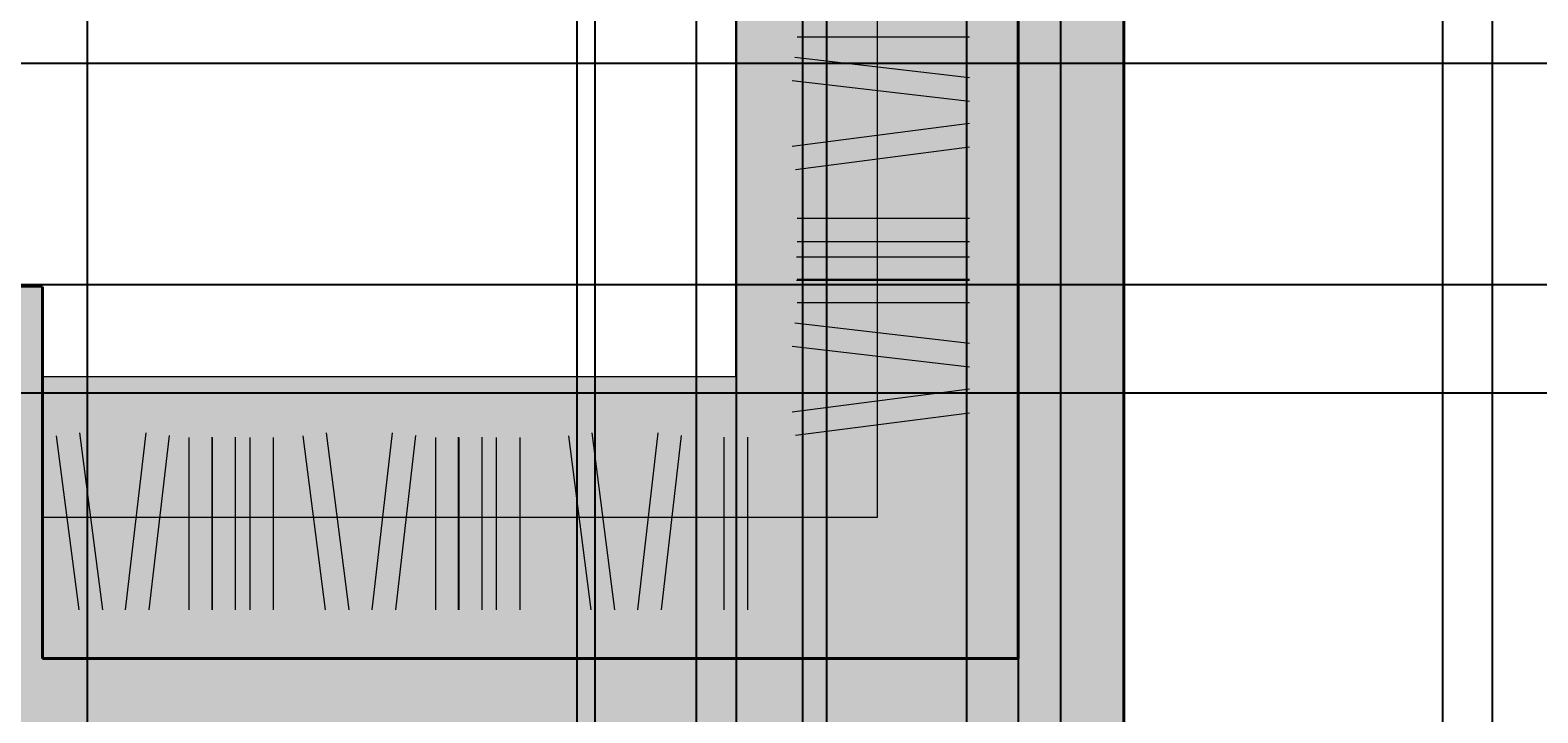
# Model space of a CAD drawing. Units: inches. Extents: x 818 to 1898, y 976 to 2364.
# Tile 42 of 96: x 1622 to 1750, y 1350 to 1409. Entities that reach past the tile are written whole.
import ezdxf

# ---------------------------------------------------------------- set-up
doc = ezdxf.new("R2010")
doc.units = ezdxf.units.IN
doc.header["$LTSCALE"] = 5
doc.header["$MEASUREMENT"] = 0
for name, color, linetype, lineweight in [('A-ANNO-DIMS', 2, 'Continuous', 18), ('A-DOOR', 3, 'Continuous', 25), ('A-FLOR-CASE', 8, 'Continuous', 18), ('A-FLOR-CASE-PATT', 33, 'Continuous', 9), ('A-WALL', 7, 'Continuous', 40)]:
    doc.layers.add(name, color=color, linetype=linetype, lineweight=lineweight)
doc.layers.add('A-WALL-PATT', color=251, linetype='Continuous', lineweight=13, true_color=0x636466)
doc.styles.get("Standard").update_dxf_attribs({"font": 'arial.ttf'})
doc.dimstyles.get("Standard").update_dxf_attribs({"dimtxt": 0.18, "dimasz": 0.18, "dimexe": 0.18, "dimexo": 0.0625, "dimgap": 0.09, "dimtad": 0, "dimtih": 1, "dimtoh": 1, "dimdec": 4, "dimzin": 0, "dimdsep": 46, "dimtxsty": 'Standard', "dimcen": 0.09, "dimadec": 0, "dimazin": 0, "dimtfac": 1, "dimtdec": 4, "dimtofl": 0, "dimtmove": 0, "dimatfit": 3, "dimfxl": 1, "dimtolj": 1, "dimtzin": 0, "dimarcsym": 0})

# ---------------------------------------------------------------- blocks, each defined once
blk = doc.blocks.new('*D71')
at = {"layer": 'A-ANNO-DIMS', "color": 0, "lineweight": -2, "ltscale": 5, "transparency": 16777216}
for p, q in [((1714.79, 2053.08), (1897.92, 2053.08)), ((1897.74, 2052.9), (1897.74, 1699.76)), ((1897.74, 1346.26), (1897.74, 1699.4)), ((1714.79, 1346.08), (1897.92, 1346.08))]:
    blk.add_line(p, q, dxfattribs=at)
at = {"layer": 'A-ANNO-DIMS', "color": 0, "ltscale": 5, "transparency": 16777216}
for points in [[(1897.71, 2052.9), (1897.77, 2052.9), (1897.74, 2053.08)], [(1897.71, 1346.26), (1897.77, 1346.26), (1897.74, 1346.08)]]:
    blk.add_solid(points, dxfattribs=at)
at = {"layer": 'Defpoints', "color": 0, "ltscale": 5, "transparency": 16777216}
for p in [(1714.73, 2053.08), (1897.74, 2053.08), (1714.73, 1346.08)]:
    blk.add_point(p, dxfattribs=at)
at = {"layer": 'A-ANNO-DIMS', "color": 0, "ltscale": 5, "transparency": 16777216, "insert": (1897.74, 1699.58), "char_height": 0.18, "attachment_point": 5}
blk.add_mtext('\\A1;707', dxfattribs=at)
blk = doc.blocks.new('*D102')
at = {"layer": 'A-ANNO-DIMS', "color": 0, "lineweight": -2, "ltscale": 5, "transparency": 16777216}
for p, q in [((1565.48, 1071.12), (1565.48, 2363.87)), ((1565.66, 2363.69), (1595.63, 2363.69)), ((1626.39, 2363.69), (1596.42, 2363.69)), ((1626.57, 1071.12), (1626.57, 2363.87))]:
    blk.add_line(p, q, dxfattribs=at)
at = {"layer": 'A-ANNO-DIMS', "color": 0, "ltscale": 5, "transparency": 16777216}
for points in [[(1565.66, 2363.72), (1565.66, 2363.66), (1565.48, 2363.69)], [(1626.39, 2363.72), (1626.39, 2363.66), (1626.57, 2363.69)]]:
    blk.add_solid(points, dxfattribs=at)
at = {"layer": 'Defpoints', "color": 0, "ltscale": 5, "transparency": 16777216}
for p in [(1626.57, 2363.69), (1565.48, 1071.06), (1626.57, 1071.06)]:
    blk.add_point(p, dxfattribs=at)
at = {"layer": 'A-ANNO-DIMS', "color": 0, "ltscale": 5, "transparency": 16777216, "insert": (1596.03, 2363.69), "char_height": 0.18, "attachment_point": 5}
blk.add_mtext('\\A1;61.09', dxfattribs=at)
blk = doc.blocks.new('*D103')
at = {"layer": 'A-ANNO-DIMS', "color": 0, "lineweight": -2, "ltscale": 5, "transparency": 16777216}
for p, q in [((1626.57, 1071.12), (1626.57, 2363.87)), ((1626.75, 2363.69), (1657.7, 2363.69)), ((1689.29, 2363.69), (1658.35, 2363.69)), ((1689.47, 1071.12), (1689.47, 2363.87))]:
    blk.add_line(p, q, dxfattribs=at)
at = {"layer": 'A-ANNO-DIMS', "color": 0, "ltscale": 5, "transparency": 16777216}
for points in [[(1626.75, 2363.72), (1626.75, 2363.66), (1626.57, 2363.69)], [(1689.29, 2363.72), (1689.29, 2363.66), (1689.47, 2363.69)]]:
    blk.add_solid(points, dxfattribs=at)
at = {"layer": 'Defpoints', "color": 0, "ltscale": 5, "transparency": 16777216}
for p in [(1689.47, 2363.69), (1626.57, 1071.06), (1689.47, 1071.06)]:
    blk.add_point(p, dxfattribs=at)
at = {"layer": 'A-ANNO-DIMS', "color": 0, "ltscale": 5, "transparency": 16777216, "insert": (1658.02, 2363.69), "char_height": 0.18, "attachment_point": 5}
blk.add_mtext('\\A1;62.9', dxfattribs=at)
blk = doc.blocks.new('*D104')
at = {"layer": 'A-ANNO-DIMS', "color": 0, "lineweight": -2, "ltscale": 5, "transparency": 16777216}
for p, q in [((1689.47, 1071.12), (1689.47, 2363.87)), ((1689.65, 2363.69), (1717.4, 2363.69)), ((1745.9, 2363.69), (1718.15, 2363.69)), ((1746.08, 1071.12), (1746.08, 2363.87))]:
    blk.add_line(p, q, dxfattribs=at)
at = {"layer": 'A-ANNO-DIMS', "color": 0, "ltscale": 5, "transparency": 16777216}
for points in [[(1689.65, 2363.72), (1689.65, 2363.66), (1689.47, 2363.69)], [(1745.9, 2363.72), (1745.9, 2363.66), (1746.08, 2363.69)]]:
    blk.add_solid(points, dxfattribs=at)
at = {"layer": 'Defpoints', "color": 0, "ltscale": 5, "transparency": 16777216}
for p in [(1746.08, 2363.69), (1689.47, 1071.06), (1746.08, 1071.06)]:
    blk.add_point(p, dxfattribs=at)
at = {"layer": 'A-ANNO-DIMS', "color": 0, "ltscale": 5, "transparency": 16777216, "insert": (1717.78, 2363.69), "char_height": 0.18, "attachment_point": 5}
blk.add_mtext('\\A1;56.61', dxfattribs=at)
blk = doc.blocks.new('*D112')
at = {"layer": 'A-ANNO-DIMS', "color": 0, "lineweight": -2, "ltscale": 5, "transparency": 16777216}
for p, q in [((1135.27, 1405.71), (1897.92, 1405.71)), ((1897.74, 1405.53), (1897.74, 1396.48)), ((1897.74, 1387.07), (1897.74, 1396.12)), ((1135.27, 1386.89), (1897.92, 1386.89))]:
    blk.add_line(p, q, dxfattribs=at)
at = {"layer": 'A-ANNO-DIMS', "color": 0, "ltscale": 5, "transparency": 16777216}
for points in [[(1897.71, 1405.53), (1897.77, 1405.53), (1897.74, 1405.71)], [(1897.71, 1387.07), (1897.77, 1387.07), (1897.74, 1386.89)]]:
    blk.add_solid(points, dxfattribs=at)
at = {"layer": 'Defpoints', "color": 0, "ltscale": 5, "transparency": 16777216}
for p in [(1135.21, 1405.71), (1135.21, 1386.89), (1897.74, 1386.89)]:
    blk.add_point(p, dxfattribs=at)
at = {"layer": 'A-ANNO-DIMS', "color": 0, "ltscale": 5, "transparency": 16777216, "insert": (1897.74, 1396.3), "char_height": 0.18, "attachment_point": 5}
blk.add_mtext('\\A1;18.824', dxfattribs=at)
blk = doc.blocks.new('*D115')
at = {"layer": 'A-ANNO-DIMS', "color": 0, "lineweight": -2, "ltscale": 5, "transparency": 16777216}
for p, q in [((1766.29, 1377.66), (818.03, 1377.66)), ((818.21, 1377.48), (818.21, 1338.26)), ((818.21, 1298.68), (818.21, 1337.9)), ((1766.29, 1298.5), (818.03, 1298.5))]:
    blk.add_line(p, q, dxfattribs=at)
at = {"layer": 'A-ANNO-DIMS', "color": 0, "ltscale": 5, "transparency": 16777216}
for points in [[(818.18, 1377.48), (818.24, 1377.48), (818.21, 1377.66)], [(818.18, 1298.68), (818.24, 1298.68), (818.21, 1298.5)]]:
    blk.add_solid(points, dxfattribs=at)
at = {"layer": 'Defpoints', "color": 0, "ltscale": 5, "transparency": 16777216}
for p in [(818.21, 1377.66), (1766.35, 1377.66), (1766.35, 1298.5)]:
    blk.add_point(p, dxfattribs=at)
at = {"layer": 'A-ANNO-DIMS', "color": 0, "ltscale": 5, "transparency": 16777216, "insert": (818.21, 1338.08), "char_height": 0.18, "attachment_point": 5}
blk.add_mtext('\\A1;79.15', dxfattribs=at)
blk = doc.blocks.new('*D116')
at = {"layer": 'A-ANNO-DIMS', "color": 0, "lineweight": -2, "ltscale": 5, "transparency": 16777216}
for p, q in [((1766.29, 1456.81), (818.03, 1456.81)), ((818.21, 1456.63), (818.21, 1417.41)), ((818.21, 1377.84), (818.21, 1417.05)), ((1766.29, 1377.66), (818.03, 1377.66))]:
    blk.add_line(p, q, dxfattribs=at)
at = {"layer": 'A-ANNO-DIMS', "color": 0, "ltscale": 5, "transparency": 16777216}
for points in [[(818.18, 1456.63), (818.24, 1456.63), (818.21, 1456.81)], [(818.18, 1377.84), (818.24, 1377.84), (818.21, 1377.66)]]:
    blk.add_solid(points, dxfattribs=at)
at = {"layer": 'Defpoints', "color": 0, "ltscale": 5, "transparency": 16777216}
for p in [(818.21, 1456.81), (1766.35, 1456.81), (1766.35, 1377.66)]:
    blk.add_point(p, dxfattribs=at)
at = {"layer": 'A-ANNO-DIMS', "color": 0, "ltscale": 5, "transparency": 16777216, "insert": (818.21, 1417.23), "char_height": 0.18, "attachment_point": 5}
blk.add_mtext('\\A1;79.15', dxfattribs=at)
blk = doc.blocks.new('*D154')
at = {"layer": 'A-ANNO-DIMS', "color": 0, "lineweight": -2, "ltscale": 5, "transparency": 16777216}
for p, q in [((1701.37, 1290.14), (1701.37, 2363.87)), ((1701.55, 2363.69), (1705.22, 2363.69)), ((1709.19, 2363.69), (1705.52, 2363.69)), ((1709.37, 1298.14), (1709.37, 2363.87))]:
    blk.add_line(p, q, dxfattribs=at)
at = {"layer": 'A-ANNO-DIMS', "color": 0, "ltscale": 5, "transparency": 16777216}
for points in [[(1701.55, 2363.72), (1701.55, 2363.66), (1701.37, 2363.69)], [(1709.19, 2363.72), (1709.19, 2363.66), (1709.37, 2363.69)]]:
    blk.add_solid(points, dxfattribs=at)
at = {"layer": 'Defpoints', "color": 0, "ltscale": 5, "transparency": 16777216}
for p in [(1709.37, 2363.69), (1709.37, 1298.08), (1701.37, 1290.08)]:
    blk.add_point(p, dxfattribs=at)
at = {"layer": 'A-ANNO-DIMS', "color": 0, "ltscale": 5, "transparency": 16777216, "insert": (1705.37, 2363.69), "char_height": 0.18, "attachment_point": 5}
blk.add_mtext('\\A1;8', dxfattribs=at)
blk = doc.blocks.new('*D178')
at = {"layer": 'A-ANNO-DIMS', "color": 0, "lineweight": -2, "ltscale": 5, "transparency": 16777216}
for p, q in [((1669.73, 1600.02), (1669.73, 975.66)), ((1705.73, 1600.02), (1705.73, 975.66)), ((1669.91, 975.84), (1687.51, 975.84)), ((1705.55, 975.84), (1687.94, 975.84))]:
    blk.add_line(p, q, dxfattribs=at)
at = {"layer": 'A-ANNO-DIMS', "color": 0, "ltscale": 5, "transparency": 16777216}
for points in [[(1669.91, 975.87), (1669.91, 975.81), (1669.73, 975.84)], [(1705.55, 975.87), (1705.55, 975.81), (1705.73, 975.84)]]:
    blk.add_solid(points, dxfattribs=at)
at = {"layer": 'Defpoints', "color": 0, "ltscale": 5, "transparency": 16777216}
for p in [(1669.73, 1600.08), (1705.73, 1600.08), (1705.73, 975.84)]:
    blk.add_point(p, dxfattribs=at)
at = {"layer": 'A-ANNO-DIMS', "color": 0, "ltscale": 5, "transparency": 16777216, "insert": (1687.73, 975.84), "char_height": 0.18, "attachment_point": 5}
blk.add_mtext('\\A1;36', dxfattribs=at)
blk = doc.blocks.new('*D180')
at = {"layer": 'A-ANNO-DIMS', "color": 0, "lineweight": -2, "ltscale": 5, "transparency": 16777216}
for p, q in [((1599.73, 1639.52), (1599.73, 975.66)), ((1669.73, 1639.52), (1669.73, 975.66)), ((1599.91, 975.84), (1634.51, 975.84)), ((1669.55, 975.84), (1634.94, 975.84))]:
    blk.add_line(p, q, dxfattribs=at)
at = {"layer": 'A-ANNO-DIMS', "color": 0, "ltscale": 5, "transparency": 16777216}
for points in [[(1599.91, 975.87), (1599.91, 975.81), (1599.73, 975.84)], [(1669.55, 975.87), (1669.55, 975.81), (1669.73, 975.84)]]:
    blk.add_solid(points, dxfattribs=at)
at = {"layer": 'Defpoints', "color": 0, "ltscale": 5, "transparency": 16777216}
for p in [(1599.73, 1639.58), (1669.73, 1639.58), (1669.73, 975.84)]:
    blk.add_point(p, dxfattribs=at)
at = {"layer": 'A-ANNO-DIMS', "color": 0, "ltscale": 5, "transparency": 16777216, "insert": (1634.73, 975.84), "char_height": 0.18, "attachment_point": 5}
blk.add_mtext('\\A1;70', dxfattribs=at)
blk = doc.blocks.new('*D183')
at = {"layer": 'A-ANNO-DIMS', "color": 0, "lineweight": -2, "ltscale": 5, "transparency": 16777216}
for p, q in [((1714.73, 1545.02), (1714.73, 975.66)), ((1741.84, 1545.02), (1741.84, 975.66)), ((1714.91, 975.84), (1727.82, 975.84)), ((1741.66, 975.84), (1728.75, 975.84))]:
    blk.add_line(p, q, dxfattribs=at)
at = {"layer": 'A-ANNO-DIMS', "color": 0, "ltscale": 5, "transparency": 16777216}
for points in [[(1714.91, 975.87), (1714.91, 975.81), (1714.73, 975.84)], [(1741.66, 975.87), (1741.66, 975.81), (1741.84, 975.84)]]:
    blk.add_solid(points, dxfattribs=at)
at = {"layer": 'Defpoints', "color": 0, "ltscale": 5, "transparency": 16777216}
for p in [(1714.73, 1545.08), (1741.84, 1545.08), (1741.84, 975.84)]:
    blk.add_point(p, dxfattribs=at)
at = {"layer": 'A-ANNO-DIMS', "color": 0, "ltscale": 5, "transparency": 16777216, "insert": (1728.28, 975.84), "char_height": 0.18, "attachment_point": 5}
blk.add_mtext('\\A1;27.116', dxfattribs=at)
blk = doc.blocks.new('*D188')
at = {"layer": 'A-ANNO-DIMS', "color": 0, "lineweight": -2, "ltscale": 5, "transparency": 16777216}
for p, q in [((1714.79, 1545.08), (1897.92, 1545.08)), ((1897.74, 1544.9), (1897.74, 1445.76)), ((1897.74, 1346.26), (1897.74, 1445.4)), ((1714.79, 1346.08), (1897.92, 1346.08))]:
    blk.add_line(p, q, dxfattribs=at)
at = {"layer": 'A-ANNO-DIMS', "color": 0, "ltscale": 5, "transparency": 16777216}
for points in [[(1897.71, 1544.9), (1897.77, 1544.9), (1897.74, 1545.08)], [(1897.71, 1346.26), (1897.77, 1346.26), (1897.74, 1346.08)]]:
    blk.add_solid(points, dxfattribs=at)
at = {"layer": 'Defpoints', "color": 0, "ltscale": 5, "transparency": 16777216}
for p in [(1714.73, 1545.08), (1897.74, 1545.08), (1714.73, 1346.08)]:
    blk.add_point(p, dxfattribs=at)
at = {"layer": 'A-ANNO-DIMS', "color": 0, "ltscale": 5, "transparency": 16777216, "insert": (1897.74, 1445.58), "char_height": 0.18, "attachment_point": 5}
blk.add_mtext('\\A1;199', dxfattribs=at)
blk = doc.blocks.new('*D195')
at = {"layer": 'A-ANNO-DIMS', "color": 0, "lineweight": -2, "ltscale": 5, "transparency": 16777216}
for p, q in [((1681.73, 1379.14), (1681.73, 2363.87)), ((1681.91, 2363.69), (1693.51, 2363.69)), ((1705.55, 2363.69), (1693.95, 2363.69)), ((1705.73, 1355.14), (1705.73, 2363.87))]:
    blk.add_line(p, q, dxfattribs=at)
at = {"layer": 'A-ANNO-DIMS', "color": 0, "ltscale": 5, "transparency": 16777216}
for points in [[(1681.91, 2363.72), (1681.91, 2363.66), (1681.73, 2363.69)], [(1705.55, 2363.72), (1705.55, 2363.66), (1705.73, 2363.69)]]:
    blk.add_solid(points, dxfattribs=at)
at = {"layer": 'Defpoints', "color": 0, "ltscale": 5, "transparency": 16777216}
for p in [(1705.73, 2363.69), (1681.73, 1379.08), (1705.73, 1355.08)]:
    blk.add_point(p, dxfattribs=at)
at = {"layer": 'A-ANNO-DIMS', "color": 0, "ltscale": 5, "transparency": 16777216, "insert": (1693.73, 2363.69), "char_height": 0.18, "attachment_point": 5}
blk.add_mtext('\\A1;24', dxfattribs=at)
blk = doc.blocks.new('*D198')
at = {"layer": 'A-ANNO-DIMS', "color": 0, "lineweight": -2, "ltscale": 5, "transparency": 16777216}
for p, q in [((1741.84, 1545.02), (1741.84, 975.66)), ((1430.73, 1346.02), (1430.73, 975.66)), ((1430.91, 975.84), (1585.91, 975.84)), ((1741.66, 975.84), (1586.66, 975.84))]:
    blk.add_line(p, q, dxfattribs=at)
at = {"layer": 'A-ANNO-DIMS', "color": 0, "ltscale": 5, "transparency": 16777216}
for points in [[(1430.91, 975.87), (1430.91, 975.81), (1430.73, 975.84)], [(1741.66, 975.87), (1741.66, 975.81), (1741.84, 975.84)]]:
    blk.add_solid(points, dxfattribs=at)
at = {"layer": 'Defpoints', "color": 0, "ltscale": 5, "transparency": 16777216}
for p in [(1741.84, 1545.08), (1430.73, 1346.08), (1741.84, 975.84)]:
    blk.add_point(p, dxfattribs=at)
at = {"layer": 'A-ANNO-DIMS', "color": 0, "ltscale": 5, "transparency": 16777216, "insert": (1586.28, 975.84), "char_height": 0.18, "attachment_point": 5}
blk.add_mtext('\\A1;311.1', dxfattribs=at)
blk = doc.blocks.new('*D199')
at = {"layer": 'A-ANNO-DIMS', "color": 0, "lineweight": -2, "ltscale": 5, "transparency": 16777216}
for p, q in [((1559.79, 1687.08), (1897.92, 1687.08)), ((1897.74, 1686.9), (1897.74, 1513.15)), ((1897.74, 1339.05), (1897.74, 1512.79)), ((1660.38, 1338.87), (1897.92, 1338.87))]:
    blk.add_line(p, q, dxfattribs=at)
at = {"layer": 'A-ANNO-DIMS', "color": 0, "ltscale": 5, "transparency": 16777216}
for points in [[(1897.71, 1686.9), (1897.77, 1686.9), (1897.74, 1687.08)], [(1897.71, 1339.05), (1897.77, 1339.05), (1897.74, 1338.87)]]:
    blk.add_solid(points, dxfattribs=at)
at = {"layer": 'Defpoints', "color": 0, "ltscale": 5, "transparency": 16777216}
for p in [(1559.73, 1687.08), (1897.74, 1687.08), (1660.31, 1338.87)]:
    blk.add_point(p, dxfattribs=at)
at = {"layer": 'A-ANNO-DIMS', "color": 0, "ltscale": 5, "transparency": 16777216, "insert": (1897.74, 1512.97), "char_height": 0.18, "attachment_point": 5}
blk.add_mtext('\\A1;348.2', dxfattribs=at)
blk = doc.blocks.new('*D200')
at = {"layer": 'A-ANNO-DIMS', "color": 0, "lineweight": -2, "ltscale": 5, "transparency": 16777216}
for p, q in [((1678.33, 1477.36), (1678.33, 975.66)), ((1705.73, 1477.36), (1705.73, 975.66)), ((1678.51, 975.84), (1691.56, 975.84)), ((1705.55, 975.84), (1692.49, 975.84))]:
    blk.add_line(p, q, dxfattribs=at)
at = {"layer": 'A-ANNO-DIMS', "color": 0, "ltscale": 5, "transparency": 16777216}
for points in [[(1678.51, 975.87), (1678.51, 975.81), (1678.33, 975.84)], [(1705.55, 975.87), (1705.55, 975.81), (1705.73, 975.84)]]:
    blk.add_solid(points, dxfattribs=at)
at = {"layer": 'Defpoints', "color": 0, "ltscale": 5, "transparency": 16777216}
for p in [(1678.33, 1477.43), (1705.73, 1477.43), (1705.73, 975.84)]:
    blk.add_point(p, dxfattribs=at)
at = {"layer": 'A-ANNO-DIMS', "color": 0, "ltscale": 5, "transparency": 16777216, "insert": (1692.03, 975.84), "char_height": 0.18, "attachment_point": 5}
blk.add_mtext('\\A1;27.395', dxfattribs=at)
blk = doc.blocks.new('*D212')
at = {"layer": 'A-ANNO-DIMS', "color": 0, "lineweight": -2, "ltscale": 5, "transparency": 16777216}
for p, q in [((1681.73, 1900.02), (1681.73, 975.66)), ((1705.73, 1876.02), (1705.73, 975.66)), ((1681.91, 975.84), (1693.51, 975.84)), ((1705.55, 975.84), (1693.95, 975.84))]:
    blk.add_line(p, q, dxfattribs=at)
at = {"layer": 'A-ANNO-DIMS', "color": 0, "ltscale": 5, "transparency": 16777216}
for points in [[(1681.91, 975.87), (1681.91, 975.81), (1681.73, 975.84)], [(1705.55, 975.87), (1705.55, 975.81), (1705.73, 975.84)]]:
    blk.add_solid(points, dxfattribs=at)
at = {"layer": 'Defpoints', "color": 0, "ltscale": 5, "transparency": 16777216}
for p in [(1681.73, 1900.08), (1705.73, 1876.08), (1705.73, 975.84)]:
    blk.add_point(p, dxfattribs=at)
at = {"layer": 'A-ANNO-DIMS', "color": 0, "ltscale": 5, "transparency": 16777216, "insert": (1693.73, 975.84), "char_height": 0.18, "attachment_point": 5}
blk.add_mtext('\\A1;24', dxfattribs=at)
blk = doc.blocks.new('*D214')
at = {"layer": 'A-ANNO-DIMS', "color": 0, "lineweight": -2, "ltscale": 5, "transparency": 16777216}
for p, q in [((1511.73, 1687.02), (1511.73, 975.66)), ((1714.73, 1687.02), (1714.73, 975.66)), ((1511.91, 975.84), (1612.93, 975.84)), ((1714.55, 975.84), (1613.52, 975.84))]:
    blk.add_line(p, q, dxfattribs=at)
at = {"layer": 'A-ANNO-DIMS', "color": 0, "ltscale": 5, "transparency": 16777216}
for points in [[(1511.91, 975.87), (1511.91, 975.81), (1511.73, 975.84)], [(1714.55, 975.87), (1714.55, 975.81), (1714.73, 975.84)]]:
    blk.add_solid(points, dxfattribs=at)
at = {"layer": 'Defpoints', "color": 0, "ltscale": 5, "transparency": 16777216}
for p in [(1511.73, 1687.08), (1714.73, 1687.08), (1714.73, 975.84)]:
    blk.add_point(p, dxfattribs=at)
at = {"layer": 'A-ANNO-DIMS', "color": 0, "ltscale": 5, "transparency": 16777216, "insert": (1613.23, 975.84), "char_height": 0.18, "attachment_point": 5}
blk.add_mtext('\\A1;203', dxfattribs=at)
blk = doc.blocks.new('*D221')
at = {"layer": 'A-ANNO-DIMS', "color": 0, "lineweight": -2, "ltscale": 5, "transparency": 16777216}
for p, q in [((1668.18, 1696.02), (1668.18, 975.66)), ((1705.73, 1696.02), (1705.73, 975.66)), ((1668.36, 975.84), (1686.56, 975.84)), ((1705.55, 975.84), (1687.35, 975.84))]:
    blk.add_line(p, q, dxfattribs=at)
at = {"layer": 'A-ANNO-DIMS', "color": 0, "ltscale": 5, "transparency": 16777216}
for points in [[(1668.36, 975.87), (1668.36, 975.81), (1668.18, 975.84)], [(1705.55, 975.87), (1705.55, 975.81), (1705.73, 975.84)]]:
    blk.add_solid(points, dxfattribs=at)
at = {"layer": 'Defpoints', "color": 0, "ltscale": 5, "transparency": 16777216}
for p in [(1668.18, 1696.08), (1705.73, 1696.08), (1705.73, 975.84)]:
    blk.add_point(p, dxfattribs=at)
at = {"layer": 'A-ANNO-DIMS', "color": 0, "ltscale": 5, "transparency": 16777216, "insert": (1686.95, 975.84), "char_height": 0.18, "attachment_point": 5}
blk.add_mtext('\\A1;37.54', dxfattribs=at)
blk = doc.blocks.new('*D228')
at = {"layer": 'A-ANNO-DIMS', "color": 0, "lineweight": -2, "ltscale": 5, "transparency": 16777216}
for p, q in [((1687.39, 1802.02), (1687.39, 975.66)), ((1705.73, 1802.02), (1705.73, 975.66)), ((1687.57, 975.84), (1696.17, 975.84)), ((1705.55, 975.84), (1696.94, 975.84))]:
    blk.add_line(p, q, dxfattribs=at)
at = {"layer": 'A-ANNO-DIMS', "color": 0, "ltscale": 5, "transparency": 16777216}
for points in [[(1687.57, 975.87), (1687.57, 975.81), (1687.39, 975.84)], [(1705.55, 975.87), (1705.55, 975.81), (1705.73, 975.84)]]:
    blk.add_solid(points, dxfattribs=at)
at = {"layer": 'Defpoints', "color": 0, "ltscale": 5, "transparency": 16777216}
for p in [(1687.39, 1802.08), (1705.73, 1802.08), (1705.73, 975.84)]:
    blk.add_point(p, dxfattribs=at)
at = {"layer": 'A-ANNO-DIMS', "color": 0, "ltscale": 5, "transparency": 16777216, "insert": (1696.56, 975.84), "char_height": 0.18, "attachment_point": 5}
blk.add_mtext('\\A1;18.33', dxfattribs=at)
blk = doc.blocks.new('*D267')
at = {"layer": 'A-ANNO-DIMS', "color": 0, "lineweight": -2, "ltscale": 5, "transparency": 16777216}
for p, q in [((1714.73, 1687.02), (1714.73, 975.66)), ((1741.84, 1687.02), (1741.84, 975.66)), ((1714.91, 975.84), (1727.82, 975.84)), ((1741.66, 975.84), (1728.75, 975.84))]:
    blk.add_line(p, q, dxfattribs=at)
at = {"layer": 'A-ANNO-DIMS', "color": 0, "ltscale": 5, "transparency": 16777216}
for points in [[(1714.91, 975.87), (1714.91, 975.81), (1714.73, 975.84)], [(1741.66, 975.87), (1741.66, 975.81), (1741.84, 975.84)]]:
    blk.add_solid(points, dxfattribs=at)
at = {"layer": 'Defpoints', "color": 0, "ltscale": 5, "transparency": 16777216}
for p in [(1714.73, 1687.08), (1741.84, 1687.08), (1741.84, 975.84)]:
    blk.add_point(p, dxfattribs=at)
at = {"layer": 'A-ANNO-DIMS', "color": 0, "ltscale": 5, "transparency": 16777216, "insert": (1728.28, 975.84), "char_height": 0.18, "attachment_point": 5}
blk.add_mtext('\\A1;27.116', dxfattribs=at)

msp = doc.modelspace()

# ---------------------------------------------------------------- hatches: boundary and pattern name
at = {"layer": 'A-FLOR-CASE-PATT', "ltscale": 5}
h = msp.add_hatch(color=256, dxfattribs=at)
h.dxf.hatch_style = 1
h.paths.add_polyline_path([(1705.7251, 1941.0782), (1681.7251, 1941.0782), (1681.7251, 1900.0782), (1599.7251, 1900.0782), (1599.7251, 1876.0782), (1705.7251, 1876.0782)])
h.paths.add_polyline_path([(1457.7252, 1409.1177), (1457.7252, 1526.6712), (1439.7252, 1526.6712), (1439.7252, 1457.5313), (1446.3307, 1457.5313), (1446.3307, 1468.9514), (1446.8307, 1470.665), (1446.8307, 1469.665), (1446.8307, 1468.9514), (1446.8307, 1456.8361), (1446.8307, 1444.7258), (1446.8307, 1443.3338), (1446.3307, 1444.7258), (1446.3307, 1456.8361), (1439.7252, 1456.8361), (1439.7252, 1355.0782), (1463.7252, 1355.0782), (1463.7252, 1367.3287), (1458.0475, 1367.3287, -0.23606798), (1457.0475, 1369.3287), (1456.0475, 1369.3287, -0.11764706), (1456.0475, 1386.3287), (1457.0475, 1386.3287, -0.23606798), (1458.0475, 1388.3287), (1463.7252, 1388.3287), (1463.7252, 1389.3211)])
h.paths.add_polyline_path([(1341.2593, 1534.0782), (1246.9377, 1534.0782), (1246.9377, 1510.0782), (1341.2593, 1510.0782)])
h.paths.add_polyline_path([(1288.8272, 1519.927), (1289.8272, 1519.927), (1290.5408, 1519.927), (1302.6561, 1519.927), (1314.7664, 1519.927), (1316.1584, 1519.927), (1314.7664, 1519.427), (1302.6561, 1519.427), (1302.6561, 1512.8214), (1301.9609, 1512.8214), (1301.9609, 1519.427), (1290.5408, 1519.427)], flags=16)
h.paths.add_polyline_path([(1377.7791, 1867.0782), (1344.5531, 1867.0782), (1344.5531, 1860.4726), (1355.9731, 1860.4726), (1357.6867, 1859.9726), (1356.6867, 1859.9726), (1355.9731, 1859.9726), (1343.8579, 1859.9726), (1331.7475, 1859.9726), (1330.3556, 1859.9726), (1331.7475, 1860.4726), (1343.8579, 1860.4726), (1343.8579, 1867.0782), (1311.3271, 1867.0782), (1311.3271, 1853.7496), (1377.7791, 1853.7496)])
h.paths.add_polyline_path([(1301.148, 1610.7299, -0.46196039), (1314.4882, 1599.3725, -0.19222541), (1311.3254, 1591.4497, 0.54791519), (1336.8832, 1607.7707, 0.92061359)])
h.paths.add_polyline_path([(1370.719, 1780.5695, 1), (1332.478, 1780.5695, 1)])
h.paths.add_polyline_path([(1705.7251, 1463.0782), (1681.7251, 1463.0782), (1681.7251, 1379.0782), (1622.7252, 1379.0782), (1622.7252, 1355.0782), (1705.7251, 1355.0782)])
h.paths.add_polyline_path([(1658.1052, 1359.2188), (1658.1786, 1359.2188), (1658.1786, 1373.8763), (1658.1052, 1373.9202)], flags=16)
h.paths.add_polyline_path([(1686.9271, 1409.9311), (1686.8832, 1409.8578), (1701.5845, 1409.8578), (1701.5845, 1409.9311)], flags=16)
h.paths.add_polyline_path([(1637.1266, 1359.2188), (1637.2, 1359.2188), (1637.2, 1373.8763), (1637.1266, 1373.9202)], flags=16)
at = {"layer": 'A-WALL-PATT', "ltscale": 5}
h = msp.add_hatch(color=256, dxfattribs=at)
h.dxf.hatch_style = 1
h.paths.add_polyline_path([(1714.7251, 1521.0782), (1705.7251, 1521.0782), (1705.7251, 1467.0782), (1654.7252, 1467.0782), (1654.7252, 1463.0782), (1705.7251, 1463.0782), (1705.7251, 1355.0782), (1622.7252, 1355.0782), (1622.7252, 1379.0782), (1622.7252, 1386.6857), (1616.7252, 1386.6857), (1616.7252, 1355.0782), (1490.9163, 1355.0782), (1490.9163, 1346.0782), (1544.7605, 1346.0782), (1544.6132, 1346.8783), (1544.6729, 1346.84), (1544.6299, 1346.7874), (1544.7605, 1346.0782), (1555.1299, 1346.0782), (1555.1299, 1341.5528), (1556.1599, 1340.8639), (1556.5281, 1338.8654), (1660.3141, 1338.8654), (1660.3141, 1346.0782), (1705.7251, 1346.0782), (1705.7251, 1345.0768), (1705.8704, 1344.58), (1705.7251, 1344.3933), (1705.7251, 1334.9904), (1705.8704, 1334.4936), (1705.7251, 1334.3068), (1705.7251, 1316.2253), (1707.3573, 1316.7694), (1707.3847, 1316.8046), (1707.3807, 1316.7771), (1705.7251, 1316.2253), (1705.7251, 1314.1392), (1705.7251, 1312.0957), (1705.8703, 1312.0739), (1705.7251, 1311.8873), (1705.7251, 1310.7121), (1706.5603, 1307.9282), (1707.8887, 1307.1831), (1714.7251, 1307.1831), (1714.7251, 1346.0782)])

# ---------------------------------------------------------------- linework, layer by layer
at = {"layer": 'A-DOOR'}
msp.add_line((1622.7252, 1386.6857), (1616.7252, 1386.6857), dxfattribs=at)
at = {"layer": 'A-FLOR-CASE'}
for p, q in [((1681.7251, 1463.0782), (1681.7251, 1379.0782)), ((1701.5845, 1407.9311), (1686.9271, 1407.9311)), ((1686.7478, 1406.2264), (1701.5845, 1404.5006)), ((1686.5168, 1404.2398), (1701.5845, 1402.4871)), ((1701.5845, 1400.5839), (1686.5199, 1398.6332)), ((1701.5845, 1398.5672), (1686.7768, 1396.6498)), ((1701.5845, 1392.5123), (1686.9271, 1392.5123)), ((1701.5845, 1390.5123), (1686.9271, 1390.5123)), ((1686.8832, 1389.2561), (1701.5845, 1389.2561)), ((1686.8832, 1387.2561), (1701.5845, 1387.2561)), ((1701.5845, 1387.3294), (1686.9271, 1387.3294)), ((1701.5845, 1385.3294), (1686.9271, 1385.3294)), ((1686.7478, 1383.6247), (1701.5845, 1381.8989)), ((1686.5168, 1381.6381), (1701.5845, 1379.8854)), ((1622.7252, 1379.0782), (1681.7251, 1379.0782)), ((1622.7252, 1355.0782), (1622.7252, 1379.0782)), ((1701.5845, 1377.9822), (1686.5199, 1376.0315)), ((1701.5845, 1375.9655), (1686.7768, 1374.0481)), ((1625.8361, 1359.2188), (1623.9187, 1374.0266)), ((1627.8528, 1359.2188), (1625.9021, 1374.2835)), ((1631.5087, 1374.2866), (1629.756, 1359.2188)), ((1633.4953, 1374.0555), (1631.7695, 1359.2188)), ((1635.2, 1359.2188), (1635.2, 1373.8763)), ((1637.1266, 1373.9202), (1637.1266, 1359.2188)), ((1637.2, 1359.2188), (1637.2, 1373.8763)), ((1639.1266, 1373.9202), (1639.1266, 1359.2188)), ((1640.3829, 1359.2188), (1640.3829, 1373.8763)), ((1642.3829, 1359.2188), (1642.3829, 1373.8763)), ((1646.8147, 1359.2188), (1644.8973, 1374.0266)), ((1648.8314, 1359.2188), (1646.8807, 1374.2835)), ((1652.4873, 1374.2866), (1650.7345, 1359.2188)), ((1654.4739, 1374.0555), (1652.748, 1359.2188)), ((1656.1786, 1359.2188), (1656.1786, 1373.8763)), ((1658.1052, 1373.9202), (1658.1052, 1359.2188)), ((1658.1786, 1359.2188), (1658.1786, 1373.8763)), ((1660.1052, 1373.9202), (1660.1052, 1359.2188)), ((1661.3614, 1359.2188), (1661.3614, 1373.8763)), ((1663.3614, 1359.2188), (1663.3614, 1373.8763)), ((1669.4164, 1359.2188), (1667.499, 1374.0266)), ((1671.4331, 1359.2188), (1669.4824, 1374.2835)), ((1675.089, 1374.2866), (1673.3362, 1359.2188)), ((1677.0756, 1374.0555), (1675.3497, 1359.2188)), ((1680.7069, 1373.9202), (1680.7069, 1359.2188)), ((1682.7069, 1373.9202), (1682.7069, 1359.2188))]:
    msp.add_line(p, q, dxfattribs=at)
msp.add_lwpolyline([(1693.7252, 1463.0782), (1693.7252, 1367.0782), (1622.7252, 1367.0782)], dxfattribs=at)
at = {"layer": 'A-WALL'}
for p, q in [((1714.7251, 1545.0782), (1714.7251, 1346.0782)), ((1705.7251, 1463.0782), (1705.7251, 1355.0782)), ((1622.7252, 1386.6857), (1622.7252, 1355.0782)), ((1622.7252, 1355.0782), (1705.7251, 1355.0782))]:
    msp.add_line(p, q, dxfattribs=at)

# ---------------------------------------------------------------- dimensions: what is measured, and where the dimension line sits
at = {"layer": 'A-ANNO-DIMS', "ltscale": 5}
for base, p1, p2, override, picture, middle in [((1626.5748, 2363.6929), (1565.4835, 1071.0552), (1626.5748, 1071.0552), {"dimdec": 2, "dimlfac": 1, "dimrnd": 0, "dimzin": 0, "dimdsep": 46, "dimlunit": 2}, '*D102', (1596.0291, 2363.6929)), ((1689.4714, 2363.6929), (1626.5748, 1071.0552), (1689.4714, 1071.0552), {"dimdec": 1, "dimlfac": 1, "dimrnd": 0, "dimzin": 0, "dimdsep": 46, "dimlunit": 2}, '*D103', (1658.0231, 2363.6929)), ((1705.7251, 2363.6929), (1681.7251, 1379.0782), (1705.7251, 1355.0782), {"dimdec": 0, "dimlfac": 1, "dimrnd": 0, "dimzin": 0, "dimdsep": 46, "dimlunit": 2}, '*D195', (1693.7251, 2363.6929)), ((1746.0831, 2363.6929), (1689.4714, 1071.0552), (1746.0831, 1071.0552), {"dimdec": 2, "dimlfac": 1, "dimrnd": 0, "dimzin": 0, "dimdsep": 46, "dimlunit": 2}, '*D104', (1717.7772, 2363.6929)), ((1709.3688, 2363.6929), (1701.3688, 1290.0782), (1709.3688, 1298.0782), {"dimdec": 0, "dimlfac": 1, "dimrnd": 0, "dimzin": 0, "dimdsep": 46, "dimlunit": 2}, '*D154', (1705.3688, 2363.6929)), ((1705.7251, 975.8433), (1681.7251, 1900.0782), (1705.7251, 1876.0782), {"dimdec": 0, "dimlfac": 1, "dimrnd": 0, "dimzin": 0, "dimdsep": 46, "dimlunit": 2}, '*D212', (1693.7251, 975.8433)), ((1705.7251, 975.8433), (1687.394, 1802.0782), (1705.7251, 1802.0782), {"dimdec": 2, "dimlfac": 1, "dimrnd": 0, "dimzin": 0, "dimdsep": 46, "dimlunit": 2}, '*D228', (1696.5596, 975.8433)), ((1705.7251, 975.8433), (1668.1841, 1696.0782), (1705.7251, 1696.0782), {"dimdec": 2, "dimlfac": 1, "dimrnd": 0, "dimzin": 0, "dimdsep": 46, "dimlunit": 2}, '*D221', (1686.9546, 975.8433)), ((1714.7251, 975.8433), (1511.7251, 1687.0782), (1714.7251, 1687.0782), {"dimdec": 0, "dimlfac": 1, "dimrnd": 0, "dimzin": 0, "dimdsep": 46, "dimlunit": 2}, '*D214', (1613.2251, 975.8433)), ((1741.8409, 975.8433), (1714.7251, 1687.0782), (1741.8409, 1687.0782), {"dimdec": 3, "dimlfac": 1, "dimrnd": 0, "dimzin": 0, "dimdsep": 46, "dimlunit": 2}, '*D267', (1728.283, 975.8433)), ((1669.7251, 975.8433), (1599.7251, 1639.5782), (1669.7251, 1639.5782), {"dimdec": 0, "dimlfac": 1, "dimrnd": 0, "dimzin": 0, "dimdsep": 46, "dimlunit": 2}, '*D180', (1634.7251, 975.8433)), ((1705.7251, 975.8433), (1669.7251, 1600.0782), (1705.7251, 1600.0782), {"dimdec": 0, "dimlfac": 1, "dimrnd": 0, "dimzin": 0, "dimdsep": 46, "dimlunit": 2}, '*D178', (1687.7251, 975.8433)), ((1741.8409, 975.8433), (1430.7251, 1346.0782), (1741.8409, 1545.0782), {"dimdec": 1, "dimlfac": 1, "dimrnd": 0, "dimzin": 0, "dimdsep": 46, "dimlunit": 2}, '*D198', (1586.283, 975.8433)), ((1741.8409, 975.8433), (1714.7251, 1545.0782), (1741.8409, 1545.0782), {"dimdec": 3, "dimlfac": 1, "dimrnd": 0, "dimzin": 0, "dimdsep": 46, "dimlunit": 2}, '*D183', (1728.283, 975.8433)), ((1705.7251, 975.8433), (1678.3302, 1477.4261), (1705.7251, 1477.4261), {"dimdec": 3, "dimlfac": 1, "dimrnd": 0, "dimzin": 0, "dimdsep": 46, "dimlunit": 2}, '*D200', (1692.0277, 975.8433))]:
    dim = msp.add_linear_dim(base=base, p1=p1, p2=p2, dimstyle='Standard', override=override, dxfattribs=at)
    dim.commit()
    dim.dimension.update_dxf_attribs({"geometry": picture, "text_midpoint": middle})
for base, p1, p2, override, picture, middle in [((1897.736, 2053.0782), (1714.7251, 1346.0782), (1714.7251, 2053.0782), {"dimdec": 0, "dimlfac": 1, "dimrnd": 0, "dimzin": 0, "dimdsep": 46, "dimlunit": 2}, '*D71', (1897.736, 1699.5782)), ((1897.736, 1687.0782), (1660.3141, 1338.8654), (1559.7251, 1687.0782), {"dimdec": 1, "dimlfac": 1, "dimrnd": 0, "dimzin": 0, "dimdsep": 46, "dimlunit": 2}, '*D199', (1897.736, 1512.9718)), ((1897.736, 1545.0782), (1714.7251, 1346.0782), (1714.7251, 1545.0782), {"dimdec": 0, "dimlfac": 1, "dimrnd": 0, "dimzin": 0, "dimdsep": 46, "dimlunit": 2}, '*D188', (1897.736, 1445.5782)), ((818.2059, 1456.8088), (1766.3524, 1377.6564), (1766.3524, 1456.8088), {"dimdec": 2, "dimlfac": 1, "dimrnd": 0, "dimzin": 0, "dimdsep": 46, "dimlunit": 2}, '*D116', (818.2059, 1417.2326)), ((1897.736, 1386.8851), (1135.2058, 1405.7088), (1135.2058, 1386.8851), {"dimdec": 3, "dimlfac": 1, "dimrnd": 0, "dimzin": 0, "dimdsep": 46, "dimlunit": 2}, '*D112', (1897.736, 1396.297)), ((818.2059, 1377.6564), (1766.3524, 1298.5041), (1766.3524, 1377.6564), {"dimdec": 2, "dimlfac": 1, "dimrnd": 0, "dimzin": 0, "dimdsep": 46, "dimlunit": 2}, '*D115', (818.2059, 1338.0803))]:
    dim = msp.add_linear_dim(base=base, p1=p1, p2=p2, angle=90, dimstyle='Standard', override=override, dxfattribs=at)
    dim.commit()
    dim.dimension.update_dxf_attribs({"geometry": picture, "text_midpoint": middle})

doc.saveas('drawing.dxf')
